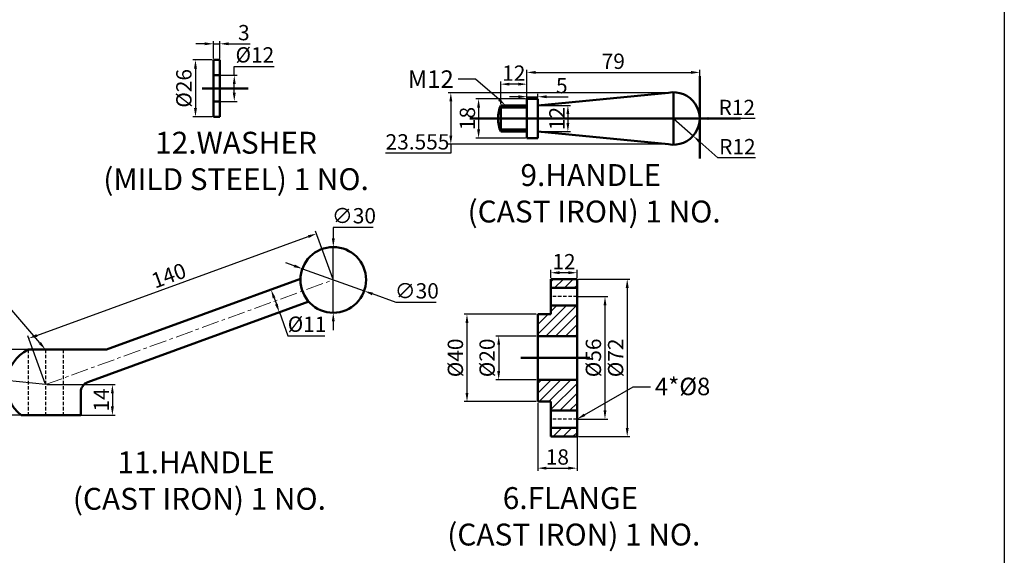
# Model space of a CAD drawing. Units: millimetres. Extents: x -66 to 1195, y -396 to 398.
# Tile 7 of 8: x 745 to 1195, y -102 to 143. Entities that reach past the tile are written whole.
import ezdxf
from ezdxf import colors
from ezdxf.entities.mleader import LeaderData, LeaderLine
from ezdxf.math import Vec2, Vec3

# ---------------------------------------------------------------- set-up
doc = ezdxf.new("R2010")
doc.units = ezdxf.units.MM
doc.header["$LTSCALE"] = 0.5
doc.linetypes.add('CENTER', pattern=[50.8, 31.75, -6.35, 6.35, -6.35])
doc.linetypes.add('HIDDEN', pattern=[9.525, 6.35, -3.175])
for name, color, linetype, lineweight in [('M-CNTR', 1, 'CENTER', 18), ('M-DIMS', 2, 'Continuous', 25), ('M-HATC', 8, 'Continuous', 18), ('M-HIDN', 3, 'HIDDEN', 25), ('M-OUTL', 7, 'Continuous', 50), ('M-TEXT', 7, 'Continuous', 25), ('M-TTLB', 7, 'Continuous', 25)]:
    doc.layers.add(name, color=color, linetype=linetype, lineweight=lineweight)
doc.styles.get("Standard").update_dxf_attribs({"font": 'arial.ttf'})
doc.dimstyles.new('ISO-25', dxfattribs={"dimtxt": 7, "dimasz": 4, "dimexe": 1.25, "dimexo": 0.625, "dimtad": 1, "dimtoh": 1, "dimtxsty": 'Standard', "dimcen": 2.5, "dimadec": 0, "dimazin": 0, "dimtfac": 1, "dimtmove": 0, "dimatfit": 3, "dimfxl": 1, "dimarcsym": 0})

# ---------------------------------------------------------------- blocks, each defined once
blk = doc.blocks.new('*D69')
at = {"layer": 'Defpoints', "color": 0, "ltscale": 0.5, "transparency": 16777216}
for p in [(836.46, 131.49), (833.46, 124.13), (836.46, 124.13)]:
    blk.add_point(p, dxfattribs=at)
at = {"layer": 'M-DIMS', "color": 0, "lineweight": -2, "ltscale": 0.5, "transparency": 16777216}
for p, q in [((829.46, 131.49), (825.46, 131.49)), ((833.46, 124.75), (833.46, 132.74)), ((833.46, 131.49), (836.46, 131.49)), ((836.46, 124.75), (836.46, 132.74)), ((840.46, 131.49), (850.29, 131.49))]:
    blk.add_line(p, q, dxfattribs=at)
at = {"layer": 'M-DIMS', "color": 0, "ltscale": 0.5, "transparency": 16777216}
for points in [[(829.46, 132.16), (829.46, 130.83), (833.46, 131.49)], [(840.46, 132.16), (840.46, 130.83), (836.46, 131.49)]]:
    blk.add_solid(points, dxfattribs=at)
at = {"layer": 'M-DIMS', "color": 0, "ltscale": 0.5, "transparency": 16777216, "insert": (847.38, 135.69), "char_height": 7, "attachment_point": 5}
blk.add_mtext('3', dxfattribs=at)
blk = doc.blocks.new('*D70')
at = {"layer": 'Defpoints', "color": 0, "ltscale": 0.5, "transparency": 16777216}
for p in [(833.46, 124.13), (825.27, 98.13), (833.46, 98.13)]:
    blk.add_point(p, dxfattribs=at)
at = {"layer": 'M-DIMS', "color": 0, "lineweight": -2, "ltscale": 0.5, "transparency": 16777216}
for p, q in [((832.84, 124.13), (824.02, 124.13)), ((825.27, 120.13), (825.27, 102.13)), ((832.84, 98.13), (824.02, 98.13))]:
    blk.add_line(p, q, dxfattribs=at)
at = {"layer": 'M-DIMS', "color": 0, "ltscale": 0.5, "transparency": 16777216}
for points in [[(824.6, 120.13), (825.93, 120.13), (825.27, 124.13)], [(824.6, 102.13), (825.93, 102.13), (825.27, 98.13)]]:
    blk.add_solid(points, dxfattribs=at)
at = {"layer": 'M-DIMS', "color": 0, "ltscale": 0.5, "transparency": 16777216, "insert": (820.87, 111.13), "char_height": 7, "attachment_point": 5, "rotation": 90}
blk.add_mtext('%%C26', dxfattribs=at)
blk = doc.blocks.new('*D71')
at = {"layer": 'Defpoints', "color": 0, "ltscale": 0.5, "transparency": 16777216}
for p in [(836.46, 117.13), (836.46, 105.13), (843.01, 105.13)]:
    blk.add_point(p, dxfattribs=at)
at = {"layer": 'M-DIMS', "color": 0, "lineweight": -2, "ltscale": 0.5, "transparency": 16777216}
for p, q in [((837.09, 117.13), (844.26, 117.13)), ((843.01, 117.13), (843.01, 121.13)), ((843.01, 121.13), (861.2, 121.13)), ((843.01, 109.13), (843.01, 113.13)), ((837.09, 105.13), (844.26, 105.13))]:
    blk.add_line(p, q, dxfattribs=at)
at = {"layer": 'M-DIMS', "color": 0, "ltscale": 0.5, "transparency": 16777216}
for points in [[(842.34, 113.13), (843.67, 113.13), (843.01, 117.13)], [(842.34, 109.13), (843.67, 109.13), (843.01, 105.13)]]:
    blk.add_solid(points, dxfattribs=at)
at = {"layer": 'M-DIMS', "color": 0, "ltscale": 0.5, "transparency": 16777216, "insert": (852.42, 125.52), "char_height": 7, "attachment_point": 5}
blk.add_mtext('%%C12', dxfattribs=at)
blk = doc.blocks.new('*D72')
at = {"layer": 'Defpoints', "color": 0, "ltscale": 0.5, "transparency": 16777216}
for p in [(880.59, 44.72), (888.28, 23.6), (756.72, -24.28)]:
    blk.add_point(p, dxfattribs=at)
at = {"layer": 'M-DIMS', "color": 0, "lineweight": -2, "ltscale": 0.5, "transparency": 16777216}
for p, q in [((888.06, 24.19), (880.16, 45.9)), ((752.79, -1.79), (876.83, 43.35)), ((756.51, -23.7), (748.6, -1.99))]:
    blk.add_line(p, q, dxfattribs=at)
at = {"layer": 'M-DIMS', "color": 0, "ltscale": 0.5, "transparency": 16777216}
for points in [[(876.6, 43.98), (877.06, 42.73), (880.59, 44.72)], [(752.56, -1.17), (753.02, -2.42), (749.03, -3.16)]]:
    blk.add_solid(points, dxfattribs=at)
at = {"layer": 'M-DIMS', "color": 0, "ltscale": 0.5, "transparency": 16777216, "insert": (813.37, 24.73), "char_height": 7, "attachment_point": 5, "rotation": 20}
blk.add_mtext('140', dxfattribs=at)
blk = doc.blocks.new('*D73')
at = {"layer": 'Defpoints', "color": 0, "ltscale": 0.5, "transparency": 16777216}
for p in [(873.28, 24), (877.04, 13.66), (863.61, 8.77)]:
    blk.add_point(p, dxfattribs=at)
at = {"layer": 'M-DIMS', "color": 0, "lineweight": -2, "ltscale": 0.5, "transparency": 16777216}
for p, q in [((872.69, 23.78), (858.67, 18.68)), ((861.21, 15.35), (862.24, 12.53)), ((876.46, 13.45), (862.43, 8.34)), ((863.61, 8.77), (867.51, -1.96)), ((867.51, -1.96), (884.43, -1.96))]:
    blk.add_line(p, q, dxfattribs=at)
at = {"layer": 'M-DIMS', "color": 0, "ltscale": 0.5, "transparency": 16777216}
for points in [[(861.84, 15.57), (860.58, 15.12), (859.84, 19.1)], [(862.86, 12.75), (861.61, 12.3), (863.61, 8.77)]]:
    blk.add_solid(points, dxfattribs=at)
at = {"layer": 'M-DIMS', "color": 0, "ltscale": 0.5, "transparency": 16777216, "insert": (876.28, 2.43), "char_height": 7, "attachment_point": 5}
blk.add_mtext('%%C11', dxfattribs=at)
blk = doc.blocks.new('*D74')
at = {"layer": 'Defpoints', "color": 0, "ltscale": 0.5, "transparency": 16777216}
for p in [(874.16, 28.67), (902.39, 18.53)]:
    blk.add_point(p, dxfattribs=at)
at = {"layer": 'M-DIMS', "color": 0, "lineweight": -2, "ltscale": 0.5, "transparency": 16777216}
for p, q in [((870.4, 30.03), (866.63, 31.38)), ((874.16, 28.67), (902.39, 18.53)), ((917.02, 13.27), (906.16, 17.17)), ((935.26, 13.27), (917.02, 13.27))]:
    blk.add_line(p, q, dxfattribs=at)
at = {"layer": 'M-DIMS', "color": 0, "ltscale": 0.5, "transparency": 16777216}
for points in [[(870.62, 30.65), (870.17, 29.4), (874.16, 28.67)], [(906.38, 17.8), (905.93, 16.55), (902.39, 18.53)]]:
    blk.add_solid(points, dxfattribs=at)
at = {"layer": 'M-DIMS', "color": 0, "ltscale": 0.5, "transparency": 16777216, "insert": (926.45, 17.67), "char_height": 7, "attachment_point": 5}
blk.add_mtext('∅30', dxfattribs=at)
blk = doc.blocks.new('*D75')
at = {"layer": 'Defpoints', "color": 0, "ltscale": 0.5, "transparency": 16777216}
for p in [(756.72, -8.28), (733.17, -38.28), (755.15, -38.28)]:
    blk.add_point(p, dxfattribs=at)
at = {"layer": 'M-DIMS', "color": 0, "lineweight": -2, "ltscale": 0.5, "transparency": 16777216}
for p, q in [((756.1, -8.28), (731.92, -8.28)), ((733.17, -12.28), (733.17, -34.28)), ((754.53, -38.28), (731.92, -38.28))]:
    blk.add_line(p, q, dxfattribs=at)
at = {"layer": 'M-DIMS', "color": 0, "ltscale": 0.5, "transparency": 16777216}
for points in [[(732.51, -12.28), (733.84, -12.28), (733.17, -8.28)], [(732.51, -34.28), (733.84, -34.28), (733.17, -38.28)]]:
    blk.add_solid(points, dxfattribs=at)
at = {"layer": 'M-DIMS', "color": 0, "ltscale": 0.5, "transparency": 16777216, "insert": (728.97, -23.28), "char_height": 7, "attachment_point": 5, "rotation": 90}
blk.add_mtext('30', dxfattribs=at)
blk = doc.blocks.new('*D76')
at = {"layer": 'Defpoints', "color": 0, "ltscale": 0.5, "transparency": 16777216}
for p in [(756.72, -24.28), (756.72, -38.28), (787.29, -38.28)]:
    blk.add_point(p, dxfattribs=at)
at = {"layer": 'M-DIMS', "color": 0, "lineweight": -2, "ltscale": 0.5, "transparency": 16777216}
for p, q in [((757.35, -24.28), (788.54, -24.28)), ((787.29, -28.28), (787.29, -34.28)), ((757.35, -38.28), (788.54, -38.28))]:
    blk.add_line(p, q, dxfattribs=at)
at = {"layer": 'M-DIMS', "color": 0, "ltscale": 0.5, "transparency": 16777216}
for points in [[(786.62, -28.28), (787.95, -28.28), (787.29, -24.28)], [(786.62, -34.28), (787.95, -34.28), (787.29, -38.28)]]:
    blk.add_solid(points, dxfattribs=at)
at = {"layer": 'M-DIMS', "color": 0, "ltscale": 0.5, "transparency": 16777216, "insert": (783.15, -31.28), "char_height": 7, "attachment_point": 5, "rotation": 90}
blk.add_mtext('14', dxfattribs=at)
blk = doc.blocks.new('*D77')
at = {"layer": 'Defpoints', "color": 0, "ltscale": 0.5, "transparency": 16777216}
for p in [(1055.8, 118.41), (976.8, 106.35), (1055.8, 106.35)]:
    blk.add_point(p, dxfattribs=at)
at = {"layer": 'M-DIMS', "color": 0, "lineweight": -2, "ltscale": 0.5, "transparency": 16777216}
for p, q in [((976.8, 106.97), (976.8, 119.66)), ((980.8, 118.41), (1051.8, 118.41)), ((1055.8, 106.97), (1055.8, 119.66))]:
    blk.add_line(p, q, dxfattribs=at)
at = {"layer": 'M-DIMS', "color": 0, "ltscale": 0.5, "transparency": 16777216}
for points in [[(980.8, 119.08), (980.8, 117.75), (976.8, 118.41)], [(1051.8, 119.08), (1051.8, 117.75), (1055.8, 118.41)]]:
    blk.add_solid(points, dxfattribs=at)
at = {"layer": 'M-DIMS', "color": 0, "ltscale": 0.5, "transparency": 16777216, "insert": (1016.3, 122.61), "char_height": 7, "attachment_point": 5}
blk.add_mtext('79', dxfattribs=at)
blk = doc.blocks.new('*D78')
at = {"layer": 'Defpoints', "color": 0, "ltscale": 0.5, "transparency": 16777216}
for p in [(976.8, 106.35), (981.8, 107.3), (981.8, 106.35)]:
    blk.add_point(p, dxfattribs=at)
at = {"layer": 'M-DIMS', "color": 0, "lineweight": -2, "ltscale": 0.5, "transparency": 16777216}
for p, q in [((976.8, 106.97), (976.8, 108.55)), ((981.8, 106.97), (981.8, 108.55)), ((972.8, 107.3), (968.8, 107.3)), ((976.8, 107.3), (981.8, 107.3)), ((985.8, 107.3), (995.69, 107.3))]:
    blk.add_line(p, q, dxfattribs=at)
at = {"layer": 'M-DIMS', "color": 0, "ltscale": 0.5, "transparency": 16777216}
for points in [[(972.8, 107.97), (972.8, 106.63), (976.8, 107.3)], [(985.8, 107.97), (985.8, 106.63), (981.8, 107.3)]]:
    blk.add_solid(points, dxfattribs=at)
at = {"layer": 'M-DIMS', "color": 0, "ltscale": 0.5, "transparency": 16777216, "insert": (992.74, 111.48), "char_height": 7, "attachment_point": 5}
blk.add_mtext('5', dxfattribs=at)
blk = doc.blocks.new('*D79')
at = {"layer": 'Defpoints', "color": 0, "ltscale": 0.5, "transparency": 16777216}
for p in [(981.8, 103.35), (981.8, 91.35), (995.54, 91.35)]:
    blk.add_point(p, dxfattribs=at)
at = {"layer": 'M-DIMS', "color": 0, "lineweight": -2, "ltscale": 0.5, "transparency": 16777216}
for p, q in [((982.42, 103.35), (996.79, 103.35)), ((995.54, 99.35), (995.54, 95.35)), ((982.42, 91.35), (996.79, 91.35))]:
    blk.add_line(p, q, dxfattribs=at)
at = {"layer": 'M-DIMS', "color": 0, "ltscale": 0.5, "transparency": 16777216}
for points in [[(994.87, 99.35), (996.2, 99.35), (995.54, 103.35)], [(994.87, 95.35), (996.2, 95.35), (995.54, 91.35)]]:
    blk.add_solid(points, dxfattribs=at)
at = {"layer": 'M-DIMS', "color": 0, "ltscale": 0.5, "transparency": 16777216, "insert": (991.4, 97.35), "char_height": 7, "attachment_point": 5, "rotation": 90}
blk.add_mtext('12', dxfattribs=at)
blk = doc.blocks.new('*D80')
at = {"layer": 'Defpoints', "color": 0, "ltscale": 0.5, "transparency": 16777216}
for p in [(976.8, 106.35), (954.7, 88.35), (976.8, 88.35)]:
    blk.add_point(p, dxfattribs=at)
at = {"layer": 'M-DIMS', "color": 0, "lineweight": -2, "ltscale": 0.5, "transparency": 16777216}
for p, q in [((976.17, 106.35), (953.45, 106.35)), ((954.7, 102.35), (954.7, 92.35)), ((976.17, 88.35), (953.45, 88.35))]:
    blk.add_line(p, q, dxfattribs=at)
at = {"layer": 'M-DIMS', "color": 0, "ltscale": 0.5, "transparency": 16777216}
for points in [[(954.04, 102.35), (955.37, 102.35), (954.7, 106.35)], [(954.04, 92.35), (955.37, 92.35), (954.7, 88.35)]]:
    blk.add_solid(points, dxfattribs=at)
at = {"layer": 'M-DIMS', "color": 0, "ltscale": 0.5, "transparency": 16777216, "insert": (950.5, 97.35), "char_height": 7, "attachment_point": 5, "rotation": 90}
blk.add_mtext('18', dxfattribs=at)
blk = doc.blocks.new('*D81')
at = {"layer": 'Defpoints', "color": 0, "ltscale": 0.5, "transparency": 16777216}
for p in [(964.8, 113.04), (964.8, 103.35), (976.8, 103.35)]:
    blk.add_point(p, dxfattribs=at)
at = {"layer": 'M-DIMS', "color": 0, "lineweight": -2, "ltscale": 0.5, "transparency": 16777216}
for p, q in [((964.8, 103.97), (964.8, 114.29)), ((972.8, 113.04), (968.8, 113.04)), ((976.8, 103.97), (976.8, 114.29))]:
    blk.add_line(p, q, dxfattribs=at)
at = {"layer": 'M-DIMS', "color": 0, "ltscale": 0.5, "transparency": 16777216}
for points in [[(968.8, 113.71), (968.8, 112.37), (964.8, 113.04)], [(972.8, 113.71), (972.8, 112.37), (976.8, 113.04)]]:
    blk.add_solid(points, dxfattribs=at)
at = {"layer": 'M-DIMS', "color": 0, "ltscale": 0.5, "transparency": 16777216, "insert": (970.8, 117.18), "char_height": 7, "attachment_point": 5}
blk.add_mtext('12', dxfattribs=at)
blk = doc.blocks.new('*D82')
at = {"layer": 'Defpoints', "color": 0, "ltscale": 0.5, "transparency": 16777216}
for p in [(1043.8, 97.35), (1052.79, 89.4)]:
    blk.add_point(p, dxfattribs=at)
at = {"layer": 'M-DIMS', "color": 0, "lineweight": -2, "ltscale": 0.5, "transparency": 16777216}
for p, q in [((1043.8, 97.35), (1052.79, 89.4)), ((1064.05, 79.44), (1055.79, 86.75)), ((1081.33, 79.44), (1064.05, 79.44))]:
    blk.add_line(p, q, dxfattribs=at)
at = {"layer": 'M-DIMS', "color": 0, "ltscale": 0.5, "transparency": 16777216}
blk.add_solid([(1056.23, 87.25), (1055.34, 86.25), (1052.79, 89.4)], dxfattribs=at)
at = {"layer": 'M-DIMS', "color": 0, "ltscale": 0.5, "transparency": 16777216, "insert": (1073, 83.58), "char_height": 7, "attachment_point": 5}
blk.add_mtext('R12', dxfattribs=at)
blk = doc.blocks.new('*D83')
at = {"layer": 'Defpoints', "color": 0, "ltscale": 0.5, "transparency": 16777216}
for p in [(999.72, 23.94), (999.72, -48.06), (1022.66, -48.06)]:
    blk.add_point(p, dxfattribs=at)
at = {"layer": 'M-DIMS', "color": 0, "lineweight": -2, "ltscale": 0.5, "transparency": 16777216}
for p, q in [((1000.34, 23.94), (1023.91, 23.94)), ((1022.66, 19.94), (1022.66, -44.06)), ((1000.34, -48.06), (1023.91, -48.06))]:
    blk.add_line(p, q, dxfattribs=at)
at = {"layer": 'M-DIMS', "color": 0, "ltscale": 0.5, "transparency": 16777216}
for points in [[(1021.99, 19.94), (1023.32, 19.94), (1022.66, 23.94)], [(1021.99, -44.06), (1023.32, -44.06), (1022.66, -48.06)]]:
    blk.add_solid(points, dxfattribs=at)
at = {"layer": 'M-DIMS', "color": 0, "ltscale": 0.5, "transparency": 16777216, "insert": (1018.26, -12.06), "char_height": 7, "attachment_point": 5, "rotation": 90}
blk.add_mtext('%%C72', dxfattribs=at)
blk = doc.blocks.new('*D84')
at = {"layer": 'Defpoints', "color": 0, "ltscale": 0.5, "transparency": 16777216}
for p in [(999.72, 15.94), (999.72, -40.06), (1012.49, -40.06)]:
    blk.add_point(p, dxfattribs=at)
at = {"layer": 'M-DIMS', "color": 0, "lineweight": -2, "ltscale": 0.5, "transparency": 16777216}
for p, q in [((1000.34, 15.94), (1013.74, 15.94)), ((1012.49, 11.94), (1012.49, -36.06)), ((1000.34, -40.06), (1013.74, -40.06))]:
    blk.add_line(p, q, dxfattribs=at)
at = {"layer": 'M-DIMS', "color": 0, "ltscale": 0.5, "transparency": 16777216}
for points in [[(1011.83, 11.94), (1013.16, 11.94), (1012.49, 15.94)], [(1011.83, -36.06), (1013.16, -36.06), (1012.49, -40.06)]]:
    blk.add_solid(points, dxfattribs=at)
at = {"layer": 'M-DIMS', "color": 0, "ltscale": 0.5, "transparency": 16777216, "insert": (1008.1, -12.06), "char_height": 7, "attachment_point": 5, "rotation": 90}
blk.add_mtext('%%C56', dxfattribs=at)
blk = doc.blocks.new('*D85')
at = {"layer": 'Defpoints', "color": 0, "ltscale": 0.5, "transparency": 16777216}
for p in [(981.72, -2.06), (963.9, -22.06), (981.72, -22.06)]:
    blk.add_point(p, dxfattribs=at)
at = {"layer": 'M-DIMS', "color": 0, "lineweight": -2, "ltscale": 0.5, "transparency": 16777216}
for p, q in [((981.09, -2.06), (962.65, -2.06)), ((963.9, -6.06), (963.9, -18.06)), ((981.09, -22.06), (962.65, -22.06))]:
    blk.add_line(p, q, dxfattribs=at)
at = {"layer": 'M-DIMS', "color": 0, "ltscale": 0.5, "transparency": 16777216}
for points in [[(963.23, -6.06), (964.57, -6.06), (963.9, -2.06)], [(963.23, -18.06), (964.57, -18.06), (963.9, -22.06)]]:
    blk.add_solid(points, dxfattribs=at)
at = {"layer": 'M-DIMS', "color": 0, "ltscale": 0.5, "transparency": 16777216, "insert": (959.51, -12.06), "char_height": 7, "attachment_point": 5, "rotation": 90}
blk.add_mtext('%%C20', dxfattribs=at)
blk = doc.blocks.new('*D86')
at = {"layer": 'Defpoints', "color": 0, "ltscale": 0.5, "transparency": 16777216}
for p in [(981.72, 7.94), (949.4, -32.06), (981.72, -32.06)]:
    blk.add_point(p, dxfattribs=at)
at = {"layer": 'M-DIMS', "color": 0, "lineweight": -2, "ltscale": 0.5, "transparency": 16777216}
for p, q in [((981.09, 7.94), (948.15, 7.94)), ((949.4, 3.94), (949.4, -28.06)), ((981.09, -32.06), (948.15, -32.06))]:
    blk.add_line(p, q, dxfattribs=at)
at = {"layer": 'M-DIMS', "color": 0, "ltscale": 0.5, "transparency": 16777216}
for points in [[(948.73, 3.94), (950.06, 3.94), (949.4, 7.94)], [(948.73, -28.06), (950.06, -28.06), (949.4, -32.06)]]:
    blk.add_solid(points, dxfattribs=at)
at = {"layer": 'M-DIMS', "color": 0, "ltscale": 0.5, "transparency": 16777216, "insert": (945, -12.06), "char_height": 7, "width": 10.4793, "attachment_point": 5, "rotation": 90}
blk.add_mtext('%%C40', dxfattribs=at)
blk = doc.blocks.new('*D87')
at = {"layer": 'Defpoints', "color": 0, "ltscale": 0.5, "transparency": 16777216}
for p in [(981.72, -32.06), (999.72, -32.06), (999.72, -62.46)]:
    blk.add_point(p, dxfattribs=at)
at = {"layer": 'M-DIMS', "color": 0, "lineweight": -2, "ltscale": 0.5, "transparency": 16777216}
for p, q in [((981.72, -32.69), (981.72, -63.71)), ((999.72, -32.69), (999.72, -63.71)), ((985.72, -62.46), (995.72, -62.46))]:
    blk.add_line(p, q, dxfattribs=at)
at = {"layer": 'M-DIMS', "color": 0, "ltscale": 0.5, "transparency": 16777216}
for points in [[(985.72, -61.79), (985.72, -63.13), (981.72, -62.46)], [(995.72, -61.79), (995.72, -63.13), (999.72, -62.46)]]:
    blk.add_solid(points, dxfattribs=at)
at = {"layer": 'M-DIMS', "color": 0, "ltscale": 0.5, "transparency": 16777216, "insert": (990.72, -58.26), "char_height": 7, "attachment_point": 5}
blk.add_mtext('18', dxfattribs=at)
blk = doc.blocks.new('*D88')
at = {"layer": 'Defpoints', "color": 0, "ltscale": 0.5, "transparency": 16777216}
for p in [(987.72, 26.86), (987.72, 23.94), (999.72, 23.94)]:
    blk.add_point(p, dxfattribs=at)
at = {"layer": 'M-DIMS', "color": 0, "lineweight": -2, "ltscale": 0.5, "transparency": 16777216}
for p, q in [((987.72, 24.56), (987.72, 28.11)), ((999.72, 24.56), (999.72, 28.11)), ((995.72, 26.86), (991.72, 26.86))]:
    blk.add_line(p, q, dxfattribs=at)
at = {"layer": 'M-DIMS', "color": 0, "ltscale": 0.5, "transparency": 16777216}
for points in [[(991.72, 27.53), (991.72, 26.2), (987.72, 26.86)], [(995.72, 27.53), (995.72, 26.2), (999.72, 26.86)]]:
    blk.add_solid(points, dxfattribs=at)
at = {"layer": 'M-DIMS', "color": 0, "ltscale": 0.5, "transparency": 16777216, "insert": (993.72, 31), "char_height": 7, "attachment_point": 5}
blk.add_mtext('12', dxfattribs=at)
blk = doc.blocks.new('*D108')
at = {"layer": 'Defpoints', "color": 0, "ltscale": 0.5, "transparency": 16777216}
for p in [(1041.5, 109.13), (942.01, 85.57), (1041.5, 85.57)]:
    blk.add_point(p, dxfattribs=at)
at = {"layer": 'M-DIMS', "color": 0, "lineweight": -2, "ltscale": 0.5, "transparency": 16777216}
for p, q in [((1040.87, 109.13), (940.76, 109.13)), ((942.01, 105.13), (942.01, 89.57)), ((1040.87, 85.57), (940.76, 85.57)), ((942.01, 85.57), (942.01, 81.57)), ((942.01, 81.57), (912.16, 81.57))]:
    blk.add_line(p, q, dxfattribs=at)
at = {"layer": 'M-DIMS', "color": 0, "ltscale": 0.5, "transparency": 16777216}
for points in [[(941.35, 105.13), (942.68, 105.13), (942.01, 109.13)], [(941.35, 89.57), (942.68, 89.57), (942.01, 85.57)]]:
    blk.add_solid(points, dxfattribs=at)
at = {"layer": 'M-DIMS', "color": 0, "ltscale": 0.5, "transparency": 16777216, "insert": (926.77, 85.77), "char_height": 7, "attachment_point": 5}
blk.add_mtext('23.555', dxfattribs=at)
blk = doc.blocks.new('*D130')
at = {"layer": 'Defpoints', "color": 0, "ltscale": 0.5, "transparency": 16777216}
for p in [(1043.8, 97.35), (1055.8, 97.35)]:
    blk.add_point(p, dxfattribs=at)
at = {"layer": 'M-DIMS', "color": 0, "lineweight": -2, "ltscale": 0.5, "transparency": 16777216}
for p, q in [((1043.8, 97.35), (1055.8, 97.35)), ((1063.8, 97.35), (1059.8, 97.35)), ((1081.08, 97.35), (1063.8, 97.35))]:
    blk.add_line(p, q, dxfattribs=at)
at = {"layer": 'M-DIMS', "color": 0, "ltscale": 0.5, "transparency": 16777216}
blk.add_solid([(1059.8, 98.02), (1059.8, 96.68), (1055.8, 97.35)], dxfattribs=at)
at = {"layer": 'M-DIMS', "color": 0, "ltscale": 0.5, "transparency": 16777216, "insert": (1072.75, 101.49), "char_height": 7, "attachment_point": 5}
blk.add_mtext('R12', dxfattribs=at)
blk = doc.blocks.new('*D131')
at = {"layer": 'Defpoints', "color": 0, "ltscale": 0.5, "transparency": 16777216}
for p in [(888.28, 38.6), (888.27, 8.6)]:
    blk.add_point(p, dxfattribs=at)
at = {"layer": 'M-DIMS', "color": 0, "lineweight": -2, "ltscale": 0.5, "transparency": 16777216}
for p, q in [((906.53, 47.6), (888.28, 47.6)), ((888.28, 47.6), (888.28, 42.6)), ((888.27, 8.6), (888.28, 38.6)), ((888.27, 4.6), (888.27, 0.6))]:
    blk.add_line(p, q, dxfattribs=at)
at = {"layer": 'M-DIMS', "color": 0, "ltscale": 0.5, "transparency": 16777216}
for points in [[(887.61, 42.6), (888.95, 42.6), (888.28, 38.6)], [(887.61, 4.6), (888.94, 4.6), (888.27, 8.6)]]:
    blk.add_solid(points, dxfattribs=at)
at = {"layer": 'M-DIMS', "color": 0, "ltscale": 0.5, "transparency": 16777216, "insert": (897.72, 52), "char_height": 7, "attachment_point": 5}
blk.add_mtext('∅30', dxfattribs=at)
blk = doc.blocks.new('*D132')
at = {"layer": 'Defpoints', "color": 0, "ltscale": 0.5, "transparency": 16777216}
for p in [(738.93, -22.42), (756.72, -24.28)]:
    blk.add_point(p, dxfattribs=at)
at = {"layer": 'M-DIMS', "color": 0, "lineweight": -2, "ltscale": 0.5, "transparency": 16777216}
for p, q in [((697.29, -21.3), (728.25, -21.3)), ((728.25, -21.3), (734.95, -22)), ((756.72, -24.28), (738.93, -22.42))]:
    blk.add_line(p, q, dxfattribs=at)
at = {"layer": 'M-DIMS', "color": 0, "ltscale": 0.5, "transparency": 16777216}
blk.add_solid([(735.02, -21.34), (734.88, -22.67), (738.93, -22.42)], dxfattribs=at)
at = {"layer": 'M-DIMS', "color": 0, "ltscale": 0.5, "transparency": 16777216, "insert": (712.46, -17.1), "char_height": 7, "attachment_point": 5}
blk.add_mtext('R17.89', dxfattribs=at)

msp = doc.modelspace()

# ---------------------------------------------------------------- hatches: boundary and pattern name
at = {"layer": 'M-HATC', "ltscale": 0.5}
h = msp.add_hatch(dxfattribs=at)
h.set_pattern_fill('ANSI31', color=256)
h.set_pattern_definition([(45, (-350.938, -238.359), (-2.245064, 2.245064), [])])
h.paths.add_polyline_path([(999.7189, 11.9364), (987.7189, 11.9364), (987.7189, 7.9364), (981.7189, 7.9364), (981.7189, -2.0636), (999.7189, -2.0636)])
h.paths.add_polyline_path([(999.7189, 19.9364), (999.7189, 23.9364), (987.7189, 23.9364), (987.7189, 19.9364)])
h.paths.add_polyline_path([(999.7189, -48.0636), (999.7189, -44.0636), (987.7189, -44.0636), (987.7189, -48.0636)])
h.paths.add_polyline_path([(999.7189, -36.0636), (999.7189, -22.0636), (981.7189, -22.0636), (981.7189, -32.0636), (987.7189, -32.0636), (987.7189, -36.0636)])

# ---------------------------------------------------------------- linework, layer by layer
at = {"layer": 'M-CNTR', "ltscale": 0.5}
msp.add_line((756.72, -24.2825), (888.277, 23.6003), dxfattribs=at)
at = {"layer": 'M-HIDN', "ltscale": 0.5}
for p, q in [((999.7189, 15.9364), (987.7189, 15.9364)), ((748.72, -8.2825), (748.72, -38.2825)), ((756.72, -8.2825), (756.72, -38.2825)), ((764.72, -8.2825), (764.72, -38.2825)), ((999.7189, -40.0636), (987.7189, -40.0636))]:
    msp.add_line(p, q, dxfattribs=at)
at = {"layer": 'M-OUTL', "ltscale": 0.5}
for p, q in [((833.4608, 124.1253), (833.4608, 98.1253)), ((836.4608, 124.1253), (833.4608, 124.1253)), ((836.4608, 98.1253), (836.4608, 124.1253)), ((833.4608, 117.1253), (836.4608, 117.1253)), ((1055.7994, 79.0792), (1055.7994, 116.6421)), ((828.3907, 111.1253), (849.3127, 111.1253)), ((1041.4983, 109.125), (981.7994, 103.3477)), ((1043.7994, 109.3477), (1043.7994, 85.3477)), ((833.4608, 105.1253), (836.4608, 105.1253)), ((976.7994, 106.3477), (976.7994, 88.3477)), ((981.7994, 106.3477), (976.7994, 106.3477)), ((981.7994, 88.3477), (981.7994, 106.3477)), ((976.7994, 103.3477), (964.7994, 103.3477)), ((964.7994, 103.3477), (964.7994, 91.3477)), ((976.7994, 102.3477), (964.7994, 102.3477)), ((976.7994, 91.3477), (976.7994, 103.3477)), ((833.4608, 98.1253), (836.4608, 98.1253)), ((950.663, 97.3477), (1074.4481, 97.3477)), ((964.7994, 92.3477), (976.7994, 92.3477)), ((964.7994, 91.3477), (976.7994, 91.3477)), ((981.7994, 91.3477), (1041.4983, 85.5704)), ((976.7994, 88.3477), (981.7994, 88.3477)), ((784.5988, -8.2825), (873.2822, 23.9956)), ((987.7189, 23.9364), (999.7189, 23.9364)), ((987.7189, 7.9364), (987.7189, 23.9364)), ((999.7189, 23.9364), (999.7189, -48.0636)), ((999.7189, 19.9364), (987.7189, 19.9364)), ((776.0909, -23.0851), (877.0444, 13.659)), ((999.7189, 11.9364), (987.7189, 11.9364)), ((981.7189, -32.0636), (981.7189, 7.9364)), ((987.7189, 7.9364), (981.7189, 7.9364)), ((999.7189, -2.0636), (981.7189, -2.0636)), ((764.72, -8.2825), (748.72, -8.2825)), ((764.72, -8.2825), (784.5988, -8.2825)), ((1005.5794, -12.0636), (974.0672, -12.0636)), ((999.7189, -22.0636), (981.7189, -22.0636)), ((772.801, -38.2825), (772.801, -27.7836)), ((987.7189, -32.0636), (981.7189, -32.0636)), ((987.7189, -48.0636), (987.7189, -32.0636)), ((764.72, -38.2825), (745.5845, -38.2825)), ((764.72, -38.2825), (772.801, -38.2825)), ((999.7189, -36.0636), (987.7189, -36.0636)), ((999.7189, -44.0636), (987.7189, -44.0636)), ((999.7189, -48.0636), (987.7189, -48.0636))]:
    msp.add_line(p, q, dxfattribs=at)
msp.add_circle((888.277, 23.6003), 15, dxfattribs=at)
for centre, radius, start, end in [((1043.7994, 97.3477), 12, 258.94492, 101.05508), ((979.4121, 97.3477), 15.7966, 157.676891, 202.323109), ((756.72, -24.2825), 17.8885, 116.565051, 231.501439), ((777.801, -27.7836), 5, 110, 180)]:
    msp.add_arc(centre, radius, start, end, dxfattribs=at)
at = {"layer": 'M-TTLB', "ltscale": 0.5}
msp.add_lwpolyline([(-66.4176, 397.641), (1195.0519, 397.641), (1195.0519, -395.6964), (-66.4176, -395.6964)], close=True, dxfattribs=at)

# ---------------------------------------------------------------- texts
at = {"layer": 'M-TEXT', "ltscale": 0.5, "char_height": 10, "attachment_point": 1}
for s, width, insert in [('\\pxqc;12.WASHER \\P(MILD STEEL) 1 NO.', 203.992441, (741.8301, 91.2784)), ('\\pxqc;9.HANDLE \\P (CAST IRON) 1 NO.', 191.333714, (910.3217, 76.5003)), ('\\pxqc;11.HANDLE \\P (CAST IRON) 1 NO.', 191.333714, (729.8685, -54.8073)), ('\\pxqc;6.FLANGE\\P (CAST IRON) 1 NO.', 191.333714, (901.026, -71.1435))]:
    msp.add_mtext_dynamic_manual_height_columns(s, width=width, gutter_width=12.5, heights=[0], dxfattribs=dict(at, insert=insert))

# ---------------------------------------------------------------- dimensions: what is measured, and where the dimension line sits
at = {"layer": 'M-DIMS', "ltscale": 0.5}
for base, p1, p2, picture, middle in [((836.4608, 131.4917), (833.4608, 124.1253), (836.4608, 124.1253), '*D69', (847.3778, 135.6931)), ((1055.7994, 118.4119), (976.7994, 106.3477), (1055.7994, 106.3477), '*D77', (1016.2994, 122.6109)), ((964.7994, 113.0401), (976.7994, 103.3477), (964.7994, 103.3477), '*D81', (970.7994, 117.1794)), ((981.7994, 107.2991), (976.7994, 106.3477), (981.7994, 106.3477), '*D78', (992.745, 111.4838)), ((987.7189, 26.8634), (999.7189, 23.9364), (987.7189, 23.9364), '*D88', (993.7189, 31.0028)), ((999.7189, -62.4615), (981.7189, -32.0636), (999.7189, -32.0636), '*D87', (990.7189, -58.2624))]:
    dim = msp.add_linear_dim(base=base, p1=p1, p2=p2, dimstyle='ISO-25', override={"dimclrd": 0, "dimclre": 0, "dimclrt": 0}, dxfattribs=at)
    dim.commit()
    dim.dimension.update_dxf_attribs({"geometry": picture, "text_midpoint": middle})
for base, p1, p2, angle, picture, middle, dimtype in [((843.006, 105.1253), (836.4608, 117.1253), (836.4608, 105.1253), 90, '*D71', (852.4168, 121.1253), 160), ((863.6055, 8.7676), (873.2822, 23.9956), (877.0444, 13.659), 290, '*D73', (876.2828, -1.9647), 161)]:
    dim = msp.add_linear_dim(base=base, p1=p1, p2=p2, angle=angle, text='%%C<>', dimstyle='ISO-25', override={"dimclrd": 0, "dimclre": 0, "dimclrt": 0}, dxfattribs=at)
    dim.commit()
    dim.dimension.update_dxf_attribs({"geometry": picture, "text_midpoint": middle, "dimtype": dimtype})
for base, p1, p2, picture, middle in [((825.2673, 98.1253), (833.4608, 124.1253), (833.4608, 98.1253), '*D70', (820.8725, 111.1253)), ((1022.6576, -48.0636), (999.7189, 23.9364), (999.7189, -48.0636), '*D83', (1018.2628, -12.0636)), ((1012.4924, -40.0636), (999.7189, 15.9364), (999.7189, -40.0636), '*D84', (1008.0976, -12.0636)), ((949.3964, -32.0636), (981.7189, 7.9364), (981.7189, -32.0636), '*D86', (945.0017, -12.0636)), ((963.9001, -22.0636), (981.7189, -2.0636), (981.7189, -22.0636), '*D85', (959.5053, -12.0636))]:
    dim = msp.add_linear_dim(base=base, p1=p1, p2=p2, angle=90, text='%%C<>', dimstyle='ISO-25', override={"dimclrd": 0, "dimclre": 0, "dimclrt": 0}, dxfattribs=at)
    dim.commit()
    dim.dimension.update_dxf_attribs({"geometry": picture, "text_midpoint": middle})
for base, p1, p2, override, picture, middle in [((942.013, 85.5704), (1041.4983, 109.125), (1041.4983, 85.5704), {"dimdec": 3, "dimlfac": 1, "dimrnd": 0, "dimzin": 0, "dimdsep": 46, "dimlunit": 2}, '*D108', (926.7721, 85.7718)), ((954.702, 88.3477), (976.7994, 106.3477), (976.7994, 88.3477), {"dimclrd": 0, "dimclre": 0, "dimclrt": 0}, '*D80', (950.503, 97.3477)), ((995.5359, 91.3477), (981.7994, 103.3477), (981.7994, 91.3477), {"dimclrd": 0, "dimclre": 0, "dimclrt": 0}, '*D79', (991.3965, 97.3477)), ((733.173, -38.2825), (756.72, -8.2825), (755.1523, -38.2825), {"dimclrd": 0, "dimclre": 0, "dimclrt": 0}, '*D75', (728.9716, -23.2825)), ((787.2851, -38.2825), (756.72, -24.2825), (756.72, -38.2825), {"dimclrd": 0, "dimclre": 0, "dimclrt": 0}, '*D76', (783.1458, -31.2825))]:
    dim = msp.add_linear_dim(base=base, p1=p1, p2=p2, angle=90, dimstyle='ISO-25', override=override, dxfattribs=at)
    dim.commit()
    dim.dimension.update_dxf_attribs({"geometry": picture, "text_midpoint": middle})
for mpoint, override, picture, middle in [((1055.7994, 97.35), {"dimdec": 0, "dimlfac": 1, "dimrnd": 0, "dimzin": 0, "dimdsep": 46, "dimlunit": 2}, '*D130', (1072.7518, 101.4909)), ((1052.7891, 89.3988), {"dimclrd": 0, "dimclre": 0, "dimclrt": 0}, '*D82', (1073.0002, 83.5831))]:
    dim = msp.add_radius_dim(center=(1043.7994, 97.3477), mpoint=mpoint, dimstyle='ISO-25', override=override, dxfattribs=at)
    dim.commit()
    dim.dimension.update_dxf_attribs({"geometry": picture, "text_midpoint": middle})
dim = msp.add_diameter_dim_2p(p1=(888.274, 8.6003), p2=(888.28, 38.6003), dimstyle='ISO-25', override={"dimdec": 0, "dimlfac": 1, "dimrnd": 0, "dimzin": 0, "dimdsep": 46, "dimlunit": 2}, dxfattribs=at)
dim.commit()
dim.dimension.update_dxf_attribs({"geometry": '*D131', "text_midpoint": (897.7165, 47.6003), "dimtype": 163})
dim = msp.add_aligned_dim(p1=(756.72, -24.2825), p2=(888.277, 23.6003), distance=22.4772, dimstyle='ISO-25', override={"dimclrd": 0, "dimclre": 0, "dimclrt": 0}, dxfattribs=at)
dim.commit()
dim.dimension.update_dxf_attribs({"geometry": '*D72', "text_midpoint": (813.3747, 24.7263)})
dim = msp.add_diameter_dim_2p(p1=(874.1609, 28.6733), p2=(902.3931, 18.5273), dimstyle='ISO-25', override={"dimclrd": 0, "dimclre": 0, "dimclrt": 0}, dxfattribs=at)
dim.commit()
dim.dimension.update_dxf_attribs({"geometry": '*D74', "text_midpoint": (926.4517, 17.6665)})
dim = msp.add_radius_dim(center=(756.72, -24.2825), mpoint=(738.9287, -22.4199), dimstyle='ISO-25', override={"dimdec": 2, "dimlfac": 1, "dimrnd": 0, "dimzin": 0, "dimdsep": 46, "dimlunit": 2}, dxfattribs=at)
dim.commit()
dim.dimension.update_dxf_attribs({"geometry": '*D132', "text_midpoint": (728.2539, -21.3023), "dimtype": 164})

# ---------------------------------------------------------------- leaders
at = {"layer": 'M-TEXT', "ltscale": 0.5}
ml = msp.add_multileader_mtext('Standard', dxfattribs=at)
ml.set_content('M12', color=256)
ml.set_leader_properties()
ml.build(insert=Vec2(0, 0))
ctx = ml.context
ctx.base_point, ctx.char_height, ctx.plane_origin = Vec3(921.0084, 115.3542), 8, Vec3(967.047, 103.3477)
ctx.text_align_type = 2
notes = []
notes.append((ctx, [(0, (1, 1, 0), (953.3303, 115.3542), (-1, 0), 8, [(0, [(967.047, 103.3477)], 0, [])])]))
ctx.mtext.insert, ctx.mtext.alignment, ctx.mtext.flow_direction = Vec3(943.3303, 119.3542), 3, 5
ml = msp.add_multileader_mtext('Standard', dxfattribs=at)
ml.set_content('M16', color=256)
ml.set_leader_properties()
ml.build(insert=Vec2(0, 0))
ctx = ml.context
ctx.base_point, ctx.char_height, ctx.plane_origin = Vec3(705.2463, 14.0391), 8, Vec3(756.72, -8.2825)
ctx.text_align_type = 2
notes.append((ctx, [(0, (1, 1, 0), (737.6447, 14.0391), (-1, 0), 8, [(0, [(756.72, -8.2825)], 0, [])])]))
ctx.mtext.insert, ctx.mtext.alignment, ctx.mtext.flow_direction = Vec3(727.6447, 18.1073), 3, 5
ml = msp.add_multileader_mtext('Standard', dxfattribs=at)
ml.set_content('4*%%C8', color=256)
ml.set_leader_properties()
ml.build(insert=Vec2(0, 0))
ctx = ml.context
ctx.base_point, ctx.char_height, ctx.plane_origin = Vec3(1033.3225, -25.2814), 8, Vec3(999.7189, -40.0636)
notes.append((ctx, [(0, (1, 1, 0), (1025.3225, -25.2814), (1, 0), 8, [(0, [(999.7189, -40.0636)], 0, [])])]))
ctx.mtext.insert, ctx.mtext.flow_direction = Vec3(1035.3225, -21.1204), 5
for ctx, leaders in notes:
    for number, flags, end, landing, length, lines in leaders:
        leader = LeaderData()
        leader.index, (leader.has_last_leader_line, leader.has_dogleg_vector, leader.attachment_direction) = number, flags
        leader.last_leader_point, leader.dogleg_vector, leader.dogleg_length = Vec3(end), Vec3(landing), length
        for number, points, colour, breaks in lines:
            line = LeaderLine()
            line.index, line.vertices, line.color, line.breaks = number, Vec3.list(points), colors.encode_raw_color(colour), breaks
            leader.lines.append(line)
        ctx.leaders.append(leader)

doc.saveas('drawing.dxf')
